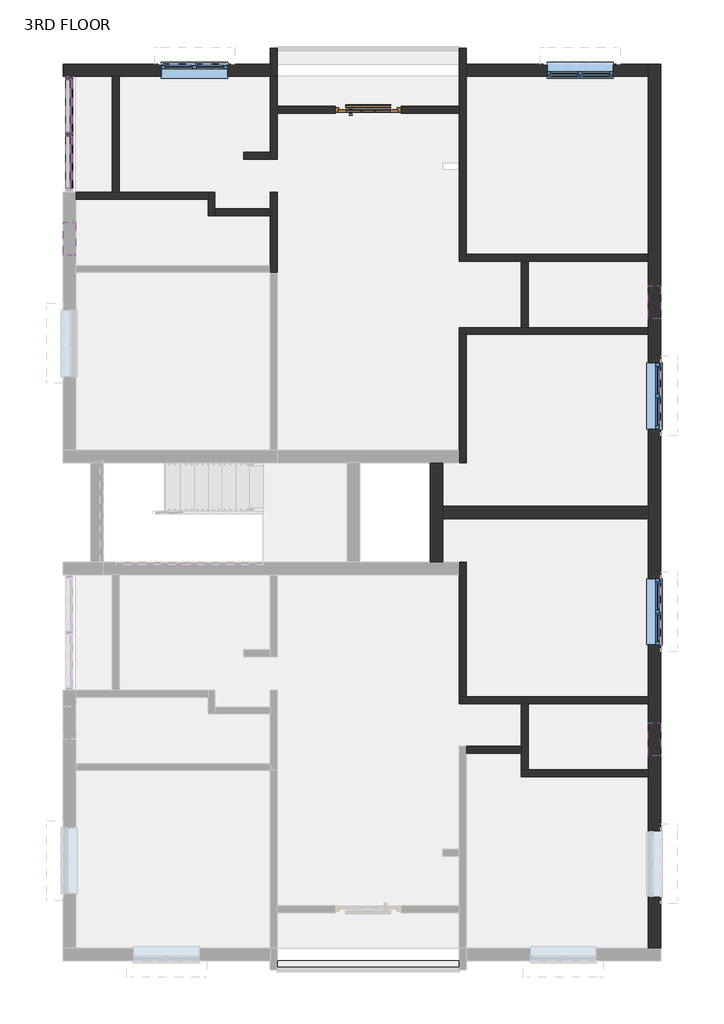
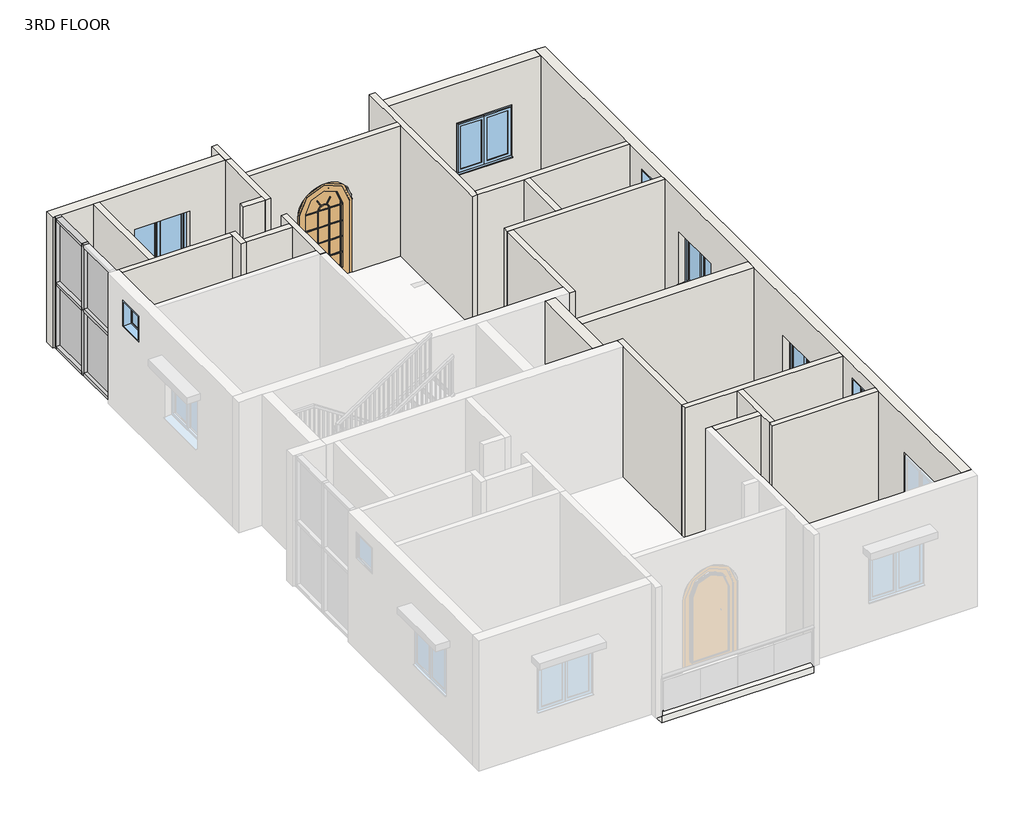
# One storey, part 2 of 4: 24 walls, 9 members, 7 windows, 4 plates, 1 door, 1 slab.
"""IFC4 building model written with IfcOpenShell, lengths in millimetres."""

from ifc_helpers import new_model, si_unit, point, frame, frame_2d, origin, place, context, project, spatial, polyline, circle_curve, trimmed, segment, composite_curve, outline, extrude, faceted_brep, transform, mapped, element, save
from components import door_arched_single_french_glass_wood_exterior_4_x_7_french_5c4dec95, member_801a2072, member_82905deb, member_88aa5c81, member_4491d118, system_panel_glazed_a8655be6, window_80340324, w2_windows_4_x_4_9dec5fc7

model = new_model("IFC4")

# Units and contexts
model_context = context("Model", 3, world=origin())
ifc_project = project(units=[si_unit("LENGTHUNIT", "METRE", prefix="MILLI")], contexts=[model_context])

# Site, building, storey
site = spatial("IfcSite", under=ifc_project)
building = spatial("IfcBuilding", under=site)
storey = spatial("IfcBuildingStorey", under=building, Name="3RD FLOOR", Elevation=12192.0)

# Door
placement = place(None, origin())
door_arched_single_french_glass_wood_exterior_4_x_7_french_shape = door_arched_single_french_glass_wood_exterior_4_x_7_french_5c4dec95(model_context)
element("IfcDoor", 1, ObjectType="Door_Arched_Single_French_Glass_Wood_Exterior : 4' x 7' french door", at=placement, inside=storey, context=model_context, shape_type="MappedRepresentation", body=[
    mapped(door_arched_single_french_glass_wood_exterior_4_x_7_french_shape, transform((-817.6012202, 12433.0309003, 12192.0), x_axis=(1.0, 0.0, 0.0), y_axis=(0.0, 1.0, 0.0), z_axis=(0.0, 0.0, 1.0))),
])

# Members
member_shape = member_801a2072(model_context)
element("IfcMember", 2, ObjectType="Rectangular Mullion : 2.5\" x 5\" rectangular", at=placement, inside=storey, context=model_context, shape_type="MappedRepresentation", body=[
    mapped(member_shape, transform((-6318.2887202, 12007.5809003, 15240.0), x_axis=(0.0, 0.0, 1.0), y_axis=(-1.0, 0.0, 0.0), z_axis=(0.0, -1.0, 0.0))),
])
element("IfcMember", 3, ObjectType="Rectangular Mullion : 2.5\" x 5\" rectangular", at=placement, inside=storey, context=model_context, shape_type="MappedRepresentation", body=[
    mapped(member_shape, transform((-6318.2887202, 12979.1309003, 12192.0), x_axis=(0.0, 0.0, -1.0), y_axis=(-1.0, 0.0, 0.0), z_axis=(0.0, 1.0, 0.0))),
])
element("IfcMember", 4, ObjectType="Rectangular Mullion : 2.5\" x 5\" rectangular", at=placement, inside=storey, context=model_context, shape_type="MappedRepresentation", body=[
    mapped(member_shape, transform((-6318.2887202, 11944.0809003, 12192.0), x_axis=(0.0, 0.0, -1.0), y_axis=(-1.0, 0.0, 0.0), z_axis=(0.0, 1.0, 0.0))),
])
member_2_shape = member_82905deb(model_context)
element("IfcMember", 5, ObjectType="Rectangular Mullion : 2.5\" x 5\" rectangular", at=placement, inside=storey, context=model_context, shape_type="MappedRepresentation", body=[
    mapped(member_2_shape, transform((-6318.2887202, 11975.8309003, 12192.0), x_axis=(0.0, -1.0, 0.0), y_axis=(-1.0, 0.0, 0.0), z_axis=(0.0, 0.0, -1.0))),
])
member_3_shape = member_88aa5c81(model_context)
element("IfcMember", 6, ObjectType="Rectangular Mullion : 2.5\" x 5\" rectangular", at=placement, inside=storey, context=model_context, shape_type="MappedRepresentation", body=[
    mapped(member_3_shape, transform((-6318.2887202, 12007.5809003, 13716.0), x_axis=(0.0, 0.0, 1.0), y_axis=(-1.0, 0.0, 0.0), z_axis=(0.0, -1.0, 0.0))),
])
element("IfcMember", 7, ObjectType="Rectangular Mullion : 2.5\" x 5\" rectangular", at=placement, inside=storey, context=model_context, shape_type="MappedRepresentation", body=[
    mapped(member_3_shape, transform((-6318.2887202, 10972.5309003, 13716.0), x_axis=(0.0, 0.0, 1.0), y_axis=(-1.0, 0.0, 0.0), z_axis=(0.0, -1.0, 0.0))),
])
element("IfcMember", 8, ObjectType="Rectangular Mullion : 2.5\" x 5\" rectangular", at=placement, inside=storey, context=model_context, shape_type="MappedRepresentation", body=[
    mapped(member_2_shape, transform((-6318.2887202, 11975.8309003, 13716.0), x_axis=(0.0, -1.0, 0.0), y_axis=(-1.0, 0.0, 0.0), z_axis=(0.0, 0.0, -1.0))),
])
member_4_shape = member_4491d118(model_context)
element("IfcMember", 9, ObjectType="Rectangular Mullion : 2.5\" x 5\" rectangular", at=placement, inside=storey, context=model_context, shape_type="MappedRepresentation", body=[
    mapped(member_4_shape, transform((-6318.2887202, 13042.6309003, 15240.0), x_axis=(0.0, 1.0, 0.0), y_axis=(-1.0, 0.0, 0.0), z_axis=(0.0, 0.0, 1.0))),
])
element("IfcMember", 10, ObjectType="Rectangular Mullion : 2.5\" x 5\" rectangular", at=placement, inside=storey, context=model_context, shape_type="MappedRepresentation", body=[
    mapped(member_4_shape, transform((-6318.2887202, 13042.6309003, 13716.0), x_axis=(0.0, 1.0, 0.0), y_axis=(-1.0, 0.0, 0.0), z_axis=(0.0, 0.0, 1.0))),
])

# Plates
system_panel_glazed_shape = system_panel_glazed_a8655be6(model_context)
element("IfcPlate", 11, ObjectType="System Panel : Glazed", at=placement, inside=storey, context=model_context, shape_type="MappedRepresentation", body=[
    mapped(system_panel_glazed_shape, transform((-6318.2887202, 12493.3559003, 12255.5), x_axis=(0.0, -1.0, 0.0), y_axis=(1.0, 0.0, 0.0), z_axis=(0.0, 0.0, 1.0))),
])
element("IfcPlate", 12, ObjectType="System Panel : Glazed", at=placement, inside=storey, context=model_context, shape_type="MappedRepresentation", body=[
    mapped(system_panel_glazed_shape, transform((-6318.2887202, 11458.3059003, 12255.5), x_axis=(0.0, -1.0, 0.0), y_axis=(1.0, 0.0, 0.0), z_axis=(0.0, 0.0, 1.0))),
])
element("IfcPlate", 13, ObjectType="System Panel : Glazed", at=placement, inside=storey, context=model_context, shape_type="MappedRepresentation", body=[
    mapped(system_panel_glazed_shape, transform((-6318.2887202, 12493.3559003, 13747.75), x_axis=(0.0, -1.0, 0.0), y_axis=(1.0, 0.0, 0.0), z_axis=(0.0, 0.0, 1.0))),
])
element("IfcPlate", 14, ObjectType="System Panel : Glazed", at=placement, inside=storey, context=model_context, shape_type="MappedRepresentation", body=[
    mapped(system_panel_glazed_shape, transform((-6318.2887202, 11458.3059003, 13747.75), x_axis=(0.0, -1.0, 0.0), y_axis=(1.0, 0.0, 0.0), z_axis=(0.0, 0.0, 1.0))),
])

# Slab
element("IfcSlab", 15, ObjectType="bathroom tiles", at=placement, inside=storey, context=model_context, shape_type="SweptSolid", body=[
    extrude(outline(polyline([(858.7987798, -3238.7690997), (858.7987798, -3403.8690997), (-2494.0012202, -3403.8690997), (-2494.0012202, -3238.7690997), (858.7987798, -3238.7690997)])), frame((0.0, 0.0, 12039.6), z_axis=(0.0, 0.0, 1.0), x_axis=(1.0, 0.0, 0.0)), (0.0, 0.0, 1.0), 152.4),
])

# Walls
element("IfcWall", 16, ObjectType="OUTER WALL 9\"", at=placement, inside=storey, context=model_context, shape_type="Brep", body=[
    faceted_brep([(4567.1987798, -3010.1690997, 12192.0), (4567.1987798, 13271.2309003, 12192.0), (4567.1987798, 13271.2309003, 15240.0), (4567.1987798, -3010.1690997, 15240.0), (4567.1987798, -844.8190997, 13192.0), (4567.1987798, -2064.0190997, 13192.0), (4567.1987798, -2064.0190997, 14411.2), (4567.1987798, -844.8190997, 14411.2), (4567.1987798, 2577.8309003, 13106.4), (4567.1987798, 2577.8309003, 14325.6), (4567.1987798, 3797.0309003, 14325.6), (4567.1987798, 3797.0309003, 13106.4), (4567.1987798, 6552.9309003, 13106.4), (4567.1987798, 6552.9309003, 14325.6), (4567.1987798, 7772.1309003, 14325.6), (4567.1987798, 7772.1309003, 13106.4), (4567.1987798, 539.4809003, 14935.2), (4567.1987798, 1149.0809003, 14935.2), (4567.1987798, 1149.0809003, 14325.6), (4567.1987798, 539.4809003, 14325.6), (4567.1987798, 8584.9309003, 14935.2), (4567.1987798, 9194.5309003, 14935.2), (4567.1987798, 9194.5309003, 14325.6), (4567.1987798, 8584.9309003, 14325.6), (4338.5987798, -3010.1690997, 12192.0), (4338.5987798, -3010.1690997, 15240.0), (4338.5987798, 152.1309003, 15240.0), (4338.5987798, 279.1309003, 15240.0), (4338.5987798, 1498.3309003, 15240.0), (4338.5987798, 1625.3309003, 15240.0), (4338.5987798, 4901.9309003, 15240.0), (4338.5987798, 5130.5309003, 15240.0), (4338.5987798, 8292.8309003, 15240.0), (4338.5987798, 8419.8309003, 15240.0), (4338.5987798, 9639.0309003, 15240.0), (4338.5987798, 9766.0309003, 15240.0), (4338.5987798, 13042.6309003, 15240.0), (4338.5987798, 13271.2309003, 15240.0), (4338.5987798, 13271.2309003, 12192.0), (4338.5987798, 13042.6309003, 12192.0), (4338.5987798, 9766.0309003, 12192.0), (4338.5987798, 9639.0309003, 12192.0), (4338.5987798, 8419.8309003, 12192.0), (4338.5987798, 8292.8309003, 12192.0), (4338.5987798, 5130.5309003, 12192.0), (4338.5987798, 4901.9309003, 12192.0), (4338.5987798, 1625.3309003, 12192.0), (4338.5987798, 1498.3309003, 12192.0), (4338.5987798, 279.1309003, 12192.0), (4338.5987798, 152.1309003, 12192.0), (4338.5987798, -844.8190997, 13192.0), (4338.5987798, -844.8190997, 14411.2), (4338.5987798, -2064.0190997, 14411.2), (4338.5987798, -2064.0190997, 13192.0), (4338.5987798, 2577.8309003, 13106.4), (4338.5987798, 3797.0309003, 13106.4), (4338.5987798, 3797.0309003, 14325.6), (4338.5987798, 2577.8309003, 14325.6), (4338.5987798, 6552.9309003, 13106.4), (4338.5987798, 7772.1309003, 13106.4), (4338.5987798, 7772.1309003, 14325.6), (4338.5987798, 6552.9309003, 14325.6), (4338.5987798, 539.4809003, 14935.2), (4338.5987798, 539.4809003, 14325.6), (4338.5987798, 1149.0809003, 14325.6), (4338.5987798, 1149.0809003, 14935.2), (4338.5987798, 8584.9309003, 14935.2), (4338.5987798, 8584.9309003, 14325.6), (4338.5987798, 9194.5309003, 14325.6), (4338.5987798, 9194.5309003, 14935.2)], [[[0, 1, 2, 3], [4, 5, 6, 7], [8, 9, 10, 11], [12, 13, 14, 15], [16, 17, 18, 19], [20, 21, 22, 23]], [[24, 25, 26, 27, 28, 29, 30, 31, 32, 33, 34, 35, 36, 37, 38, 39, 40, 41, 42, 43, 44, 45, 46, 47, 48, 49], [50, 51, 52, 53], [54, 55, 56, 57], [58, 59, 60, 61], [62, 63, 64, 65], [66, 67, 68, 69]], [[1, 0, 24, 49, 48, 47, 46, 45, 44, 43, 42, 41, 40, 39, 38]], [[3, 2, 37, 36, 35, 34, 33, 32, 31, 30, 29, 28, 27, 26, 25]], [[0, 3, 25, 24]], [[2, 1, 38, 37]], [[51, 50, 4, 7]], [[52, 51, 7, 6]], [[53, 52, 6, 5]], [[50, 53, 5, 4]], [[9, 8, 54, 57]], [[10, 9, 57, 56]], [[11, 10, 56, 55]], [[8, 11, 55, 54]], [[13, 12, 58, 61]], [[14, 13, 61, 60]], [[15, 14, 60, 59]], [[12, 15, 59, 58]], [[63, 62, 16, 19]], [[64, 63, 19, 18]], [[65, 64, 18, 17]], [[62, 65, 17, 16]], [[67, 66, 20, 23]], [[68, 67, 23, 22]], [[69, 68, 22, 21]], [[66, 69, 21, 20]]]),
])
element("IfcWall", 17, ObjectType="OUTER WALL 9\"", at=placement, inside=storey, context=model_context, shape_type="SweptSolid", body=[
    extrude(outline(polyline([(12192.0, 4338.5987798), (15240.0, 4338.5987798), (15240.0, 985.7987798), (12192.0, 985.7987798), (12192.0, 4338.5987798)]), holes=[polyline([(13106.4, 2479.7847416), (14325.6, 2479.7847416), (14325.6, 3698.9847416), (13106.4, 3698.9847416), (13106.4, 2479.7847416)])]), frame((0.0, 13042.6309003, 0.0), z_axis=(0.0, 1.0, 0.0), x_axis=(0.0, 0.0, 1.0)), (0.0, 0.0, 1.0), 228.6),
])
element("IfcWall", 18, ObjectType="OUTER WALL 9\"", at=placement, inside=storey, context=model_context, shape_type="Brep", body=[
    faceted_brep([(-2621.0012202, 13271.2309003, 12192.0), (-6432.5887202, 13271.2309003, 12192.0), (-6432.5887202, 13271.2309003, 15240.0), (-2621.0012202, 13271.2309003, 15240.0), (-3402.0512202, 13271.2309003, 13106.4), (-3402.0512202, 13271.2309003, 14325.6), (-4621.2512202, 13271.2309003, 14325.6), (-4621.2512202, 13271.2309003, 13106.4), (-2621.0012202, 13042.6309003, 12192.0), (-2621.0012202, 13042.6309003, 15240.0), (-5402.3012202, 13042.6309003, 15240.0), (-5529.3012202, 13042.6309003, 15240.0), (-6432.5887202, 13042.6309003, 15240.0), (-6432.5887202, 13042.6309003, 12192.0), (-5529.3012202, 13042.6309003, 12192.0), (-5402.3012202, 13042.6309003, 12192.0), (-3402.0512202, 13042.6309003, 13106.4), (-4621.2512202, 13042.6309003, 13106.4), (-4621.2512202, 13042.6309003, 14325.6), (-3402.0512202, 13042.6309003, 14325.6)], [[[0, 1, 2, 3], [4, 5, 6, 7]], [[8, 9, 10, 11, 12, 13, 14, 15], [16, 17, 18, 19]], [[1, 0, 8, 15, 14, 13]], [[3, 2, 12, 11, 10, 9]], [[2, 1, 13, 12]], [[5, 4, 16, 19]], [[6, 5, 19, 18]], [[7, 6, 18, 17]], [[4, 7, 17, 16]], [[0, 3, 9, 8]]]),
])
element("IfcWall", 19, ObjectType="OUTER WALL 9\"", at=placement, inside=storey, context=model_context, shape_type="Brep", body=[
    faceted_brep([(553.9987798, 4101.8309003, 12192.0), (553.9987798, 4901.9309003, 12192.0), (553.9987798, 5130.5309003, 12192.0), (553.9987798, 5930.6309003, 12192.0), (553.9987798, 5930.6309003, 15240.0), (553.9987798, 5130.5309003, 15240.0), (553.9987798, 4901.9309003, 15240.0), (553.9987798, 4101.8309003, 15240.0), (325.3987798, 4101.8309003, 12192.0), (325.3987798, 4101.8309003, 15240.0), (325.3987798, 5930.6309003, 15240.0), (325.3987798, 5930.6309003, 12192.0)], [[[0, 1, 2, 3, 4, 5, 6, 7]], [[8, 9, 10, 11]], [[3, 2, 1, 0, 8, 11]], [[7, 6, 5, 4, 10, 9]], [[0, 7, 9, 8]], [[4, 3, 11, 10]]]),
])
element("IfcWall", 20, ObjectType="OUTER WALL 9\"", at=placement, inside=storey, context=model_context, shape_type="SweptSolid", body=[
    extrude(outline(polyline([(4338.5987798, 4901.9309003), (553.9987798, 4901.9309003), (553.9987798, 5130.5309003), (4338.5987798, 5130.5309003), (4338.5987798, 4901.9309003)])), frame((0.0, 0.0, 12192.0), z_axis=(0.0, 0.0, 1.0), x_axis=(1.0, 0.0, 0.0)), (0.0, 0.0, 1.0), 3048.0),
])
element("IfcWall", 21, ObjectType="inner wall 5\"", at=placement, inside=storey, context=model_context, shape_type="SweptSolid", body=[
    extrude(outline(polyline([(-5529.3012202, 10909.0309003), (-5529.3012202, 13042.6309003), (-5402.3012202, 13042.6309003), (-5402.3012202, 10909.0309003), (-5529.3012202, 10909.0309003)])), frame((0.0, 0.0, 12192.0), z_axis=(0.0, 0.0, 1.0), x_axis=(1.0, 0.0, 0.0)), (0.0, 0.0, 1.0), 3048.0),
])
element("IfcWall", 22, ObjectType="inner wall 5\"", at=placement, inside=storey, context=model_context, shape_type="Brep", body=[
    faceted_brep([(-2621.0012202, 13042.6309003, 12192.0), (-2621.0012202, 11645.6309003, 12192.0), (-2621.0012202, 11518.6309003, 12192.0), (-2621.0012202, 11518.6309003, 15240.0), (-2621.0012202, 11645.6309003, 15240.0), (-2621.0012202, 13042.6309003, 15240.0), (-2494.0012202, 13042.6309003, 12192.0), (-2494.0012202, 13042.6309003, 15240.0), (-2494.0012202, 12496.5309003, 15240.0), (-2494.0012202, 12369.5309003, 15240.0), (-2494.0012202, 11518.6309003, 15240.0), (-2494.0012202, 11518.6309003, 12192.0), (-2494.0012202, 12369.5309003, 12192.0), (-2494.0012202, 12496.5309003, 12192.0)], [[[0, 1, 2, 3, 4, 5]], [[6, 7, 8, 9, 10, 11, 12, 13]], [[2, 1, 0, 6, 13, 12, 11]], [[5, 4, 3, 10, 9, 8, 7]], [[3, 2, 11, 10]], [[0, 5, 7, 6]]]),
])
element("IfcWall", 23, ObjectType="inner wall 5\"", at=placement, inside=storey, context=model_context, shape_type="SweptSolid", body=[
    extrude(outline(polyline([(-3103.6012202, 11645.6309003), (-2621.0012202, 11645.6309003), (-2621.0012202, 11518.6309003), (-3103.6012202, 11518.6309003), (-3103.6012202, 11645.6309003)])), frame((0.0, 0.0, 12192.0), z_axis=(0.0, 0.0, 1.0), x_axis=(1.0, 0.0, 0.0)), (0.0, 0.0, 1.0), 3048.0),
])
element("IfcWall", 24, ObjectType="inner wall 5\"", at=placement, inside=storey, context=model_context, shape_type="Brep", body=[
    faceted_brep([(-6202.4012202, 10782.0309003, 12192.0), (-3764.0012202, 10782.0309003, 12192.0), (-3764.0012202, 10782.0309003, 15240.0), (-6202.4012202, 10782.0309003, 15240.0), (-6202.4012202, 10909.0309003, 12192.0), (-6202.4012202, 10909.0309003, 15240.0), (-5529.3012202, 10909.0309003, 15240.0), (-5402.3012202, 10909.0309003, 15240.0), (-3764.0012202, 10909.0309003, 15240.0), (-3764.0012202, 10909.0309003, 12192.0), (-5402.3012202, 10909.0309003, 12192.0), (-5529.3012202, 10909.0309003, 12192.0)], [[[0, 1, 2, 3]], [[4, 5, 6, 7, 8, 9, 10, 11]], [[1, 0, 4, 11, 10, 9]], [[3, 2, 8, 7, 6, 5]], [[0, 3, 5, 4]], [[2, 1, 9, 8]]]),
])
element("IfcWall", 25, ObjectType="inner wall 5\"", at=placement, inside=storey, context=model_context, shape_type="Brep", body=[
    faceted_brep([(-3764.0012202, 10909.0309003, 12192.0), (-3764.0012202, 10782.0309003, 12192.0), (-3764.0012202, 10477.2309003, 12192.0), (-3764.0012202, 10477.2309003, 15240.0), (-3764.0012202, 10782.0309003, 15240.0), (-3764.0012202, 10909.0309003, 15240.0), (-3637.0012202, 10909.0309003, 12192.0), (-3637.0012202, 10909.0309003, 15240.0), (-3637.0012202, 10604.2309003, 15240.0), (-3637.0012202, 10477.2309003, 15240.0), (-3637.0012202, 10477.2309003, 12192.0), (-3637.0012202, 10604.2309003, 12192.0)], [[[0, 1, 2, 3, 4, 5]], [[6, 7, 8, 9, 10, 11]], [[2, 1, 0, 6, 11, 10]], [[5, 4, 3, 9, 8, 7]], [[0, 5, 7, 6]], [[3, 2, 10, 9]]]),
])
element("IfcWall", 26, ObjectType="inner wall 5\"", at=placement, inside=storey, context=model_context, shape_type="SweptSolid", body=[
    extrude(outline(polyline([(-2621.0012202, 10477.2309003), (-3637.0012202, 10477.2309003), (-3637.0012202, 10604.2309003), (-2621.0012202, 10604.2309003), (-2621.0012202, 10477.2309003)])), frame((0.0, 0.0, 12192.0), z_axis=(0.0, 0.0, 1.0), x_axis=(1.0, 0.0, 0.0)), (0.0, 0.0, 1.0), 3048.0),
])
element("IfcWall", 27, ObjectType="inner wall 5\"", at=placement, inside=storey, context=model_context, shape_type="Brep", body=[
    faceted_brep([(-2621.0012202, 10909.0309003, 12192.0), (-2621.0012202, 10604.2309003, 12192.0), (-2621.0012202, 10477.2309003, 12192.0), (-2621.0012202, 9562.8309003, 12192.0), (-2621.0012202, 9435.8309003, 12192.0), (-2621.0012202, 9435.8309003, 15240.0), (-2621.0012202, 9562.8309003, 15240.0), (-2621.0012202, 10477.2309003, 15240.0), (-2621.0012202, 10604.2309003, 15240.0), (-2621.0012202, 10909.0309003, 15240.0), (-2494.0012202, 10909.0309003, 12192.0), (-2494.0012202, 10909.0309003, 15240.0), (-2494.0012202, 9435.8309003, 15240.0), (-2494.0012202, 9435.8309003, 12192.0)], [[[0, 1, 2, 3, 4, 5, 6, 7, 8, 9]], [[10, 11, 12, 13]], [[4, 3, 2, 1, 0, 10, 13]], [[9, 8, 7, 6, 5, 12, 11]], [[0, 9, 11, 10]], [[5, 4, 13, 12]]]),
])
element("IfcWall", 28, ObjectType="inner wall 5\"", at=placement, inside=storey, context=model_context, shape_type="SweptSolid", body=[
    extrude(outline(polyline([(2001.7987798, 583.9309003), (985.7987798, 583.9309003), (985.7987798, 710.9309003), (2001.7987798, 710.9309003), (2001.7987798, 583.9309003)])), frame((0.0, 0.0, 12192.0), z_axis=(0.0, 0.0, 1.0), x_axis=(1.0, 0.0, 0.0)), (0.0, 0.0, 1.0), 3048.0),
])
element("IfcWall", 29, ObjectType="inner wall 5\"", at=placement, inside=storey, context=model_context, shape_type="Brep", body=[
    faceted_brep([(4338.5987798, 1625.3309003, 12192.0), (985.7987798, 1625.3309003, 12192.0), (858.7987798, 1625.3309003, 12192.0), (858.7987798, 1625.3309003, 15240.0), (985.7987798, 1625.3309003, 15240.0), (4338.5987798, 1625.3309003, 15240.0), (4338.5987798, 1498.3309003, 12192.0), (4338.5987798, 1498.3309003, 15240.0), (2128.7987798, 1498.3309003, 15240.0), (2001.7987798, 1498.3309003, 15240.0), (858.7987798, 1498.3309003, 15240.0), (858.7987798, 1498.3309003, 12192.0), (2001.7987798, 1498.3309003, 12192.0), (2128.7987798, 1498.3309003, 12192.0)], [[[0, 1, 2, 3, 4, 5]], [[6, 7, 8, 9, 10, 11, 12, 13]], [[2, 1, 0, 6, 13, 12, 11]], [[5, 4, 3, 10, 9, 8, 7]], [[3, 2, 11, 10]], [[0, 5, 7, 6]]]),
])
element("IfcWall", 30, ObjectType="inner wall 5\"", at=placement, inside=storey, context=model_context, shape_type="Brep", body=[
    faceted_brep([(985.7987798, 1625.3309003, 12192.0), (985.7987798, 4101.8309003, 12192.0), (985.7987798, 4101.8309003, 15240.0), (985.7987798, 1625.3309003, 15240.0), (858.7987798, 1625.3309003, 12192.0), (858.7987798, 1625.3309003, 15240.0), (858.7987798, 3873.2309003, 15240.0), (858.7987798, 4101.8309003, 15240.0), (858.7987798, 4101.8309003, 12192.0), (858.7987798, 3873.2309003, 12192.0)], [[[0, 1, 2, 3]], [[4, 5, 6, 7, 8, 9]], [[1, 0, 4, 9, 8]], [[3, 2, 7, 6, 5]], [[0, 3, 5, 4]], [[2, 1, 8, 7]]]),
])
element("IfcWall", 31, ObjectType="inner wall 5\"", at=placement, inside=storey, context=model_context, shape_type="Brep", body=[
    faceted_brep([(4338.5987798, 279.1309003, 12192.0), (2128.7987798, 279.1309003, 12192.0), (2001.7987798, 279.1309003, 12192.0), (2001.7987798, 279.1309003, 15240.0), (2128.7987798, 279.1309003, 15240.0), (4338.5987798, 279.1309003, 15240.0), (4338.5987798, 152.1309003, 12192.0), (4338.5987798, 152.1309003, 15240.0), (2001.7987798, 152.1309003, 15240.0), (2001.7987798, 152.1309003, 12192.0)], [[[0, 1, 2, 3, 4, 5]], [[6, 7, 8, 9]], [[2, 1, 0, 6, 9]], [[5, 4, 3, 8, 7]], [[0, 5, 7, 6]], [[3, 2, 9, 8]]]),
])
element("IfcWall", 32, ObjectType="inner wall 5\"", at=placement, inside=storey, context=model_context, shape_type="Brep", body=[
    faceted_brep([(2128.7987798, 279.1309003, 12192.0), (2128.7987798, 1498.3309003, 12192.0), (2128.7987798, 1498.3309003, 15240.0), (2128.7987798, 279.1309003, 15240.0), (2001.7987798, 279.1309003, 12192.0), (2001.7987798, 279.1309003, 15240.0), (2001.7987798, 583.9309003, 15240.0), (2001.7987798, 710.9309003, 15240.0), (2001.7987798, 1498.3309003, 15240.0), (2001.7987798, 1498.3309003, 12192.0), (2001.7987798, 710.9309003, 12192.0), (2001.7987798, 583.9309003, 12192.0)], [[[0, 1, 2, 3]], [[4, 5, 6, 7, 8, 9, 10, 11]], [[1, 0, 4, 11, 10, 9]], [[3, 2, 8, 7, 6, 5]], [[0, 3, 5, 4]], [[2, 1, 9, 8]]]),
])
element("IfcWall", 33, ObjectType="inner wall 5\"", at=placement, inside=storey, context=model_context, shape_type="SweptSolid", body=[
    extrude(outline(composite_curve([segment(polyline([(13870.6, -208.0012202), (12192.0, -208.0012202), (12192.0, 858.7987798), (15240.0, 858.7987798), (15240.0, -2494.0012202), (12192.0, -2494.0012202), (12192.0, -1427.2012202), (13870.6, -1427.2012202)]), True, "CONTINUOUS"), segment(trimmed(circle_curve(frame_2d((13870.6, -817.6012202)), 609.6), [point((13870.6, -1427.2012202))], [point((13870.6, -208.0012202))], True, "CARTESIAN"), True, "CONTINUOUS")], self_intersect=False)), frame((0.0, 12369.5309003, 0.0), z_axis=(0.0, 1.0, 0.0), x_axis=(0.0, 0.0, 1.0)), (0.0, 0.0, 1.0), 127.0),
])
element("IfcWall", 34, ObjectType="inner wall 5\"", at=placement, inside=storey, context=model_context, shape_type="Brep", body=[
    faceted_brep([(858.7987798, 13563.3309003, 12192.0), (858.7987798, 12496.5309003, 12192.0), (858.7987798, 12369.5309003, 12192.0), (858.7987798, 9639.0309003, 12192.0), (858.7987798, 9639.0309003, 15240.0), (858.7987798, 12369.5309003, 15240.0), (858.7987798, 12496.5309003, 15240.0), (858.7987798, 13563.3309003, 15240.0), (985.7987798, 13563.3309003, 12192.0), (985.7987798, 13563.3309003, 15240.0), (985.7987798, 13271.2309003, 15240.0), (985.7987798, 13042.6309003, 15240.0), (985.7987798, 9766.0309003, 15240.0), (985.7987798, 9639.0309003, 15240.0), (985.7987798, 9639.0309003, 12192.0), (985.7987798, 9766.0309003, 12192.0), (985.7987798, 13042.6309003, 12192.0), (985.7987798, 13271.2309003, 12192.0)], [[[0, 1, 2, 3, 4, 5, 6, 7]], [[8, 9, 10, 11, 12, 13, 14, 15, 16, 17]], [[3, 2, 1, 0, 8, 17, 16, 15, 14]], [[7, 6, 5, 4, 13, 12, 11, 10, 9]], [[0, 7, 9, 8]], [[4, 3, 14, 13]]]),
])
element("IfcWall", 35, ObjectType="inner wall 5\"", at=placement, inside=storey, context=model_context, shape_type="Brep", body=[
    faceted_brep([(4338.5987798, 9766.0309003, 12192.0), (985.7987798, 9766.0309003, 12192.0), (985.7987798, 9766.0309003, 15240.0), (4338.5987798, 9766.0309003, 15240.0), (4338.5987798, 9639.0309003, 12192.0), (4338.5987798, 9639.0309003, 15240.0), (2128.7987798, 9639.0309003, 15240.0), (2001.7987798, 9639.0309003, 15240.0), (985.7987798, 9639.0309003, 15240.0), (985.7987798, 9639.0309003, 12192.0), (2001.7987798, 9639.0309003, 12192.0), (2128.7987798, 9639.0309003, 12192.0)], [[[0, 1, 2, 3]], [[4, 5, 6, 7, 8, 9, 10, 11]], [[1, 0, 4, 11, 10, 9]], [[3, 2, 8, 7, 6, 5]], [[0, 3, 5, 4]], [[2, 1, 9, 8]]]),
])
element("IfcWall", 36, ObjectType="inner wall 5\"", at=placement, inside=storey, context=model_context, shape_type="Brep", body=[
    faceted_brep([(4338.5987798, 8419.8309003, 12192.0), (2128.7987798, 8419.8309003, 12192.0), (2001.7987798, 8419.8309003, 12192.0), (858.7987798, 8419.8309003, 12192.0), (858.7987798, 8419.8309003, 15240.0), (2001.7987798, 8419.8309003, 15240.0), (2128.7987798, 8419.8309003, 15240.0), (4338.5987798, 8419.8309003, 15240.0), (4338.5987798, 8292.8309003, 12192.0), (4338.5987798, 8292.8309003, 15240.0), (985.7987798, 8292.8309003, 15240.0), (858.7987798, 8292.8309003, 15240.0), (858.7987798, 8292.8309003, 12192.0), (985.7987798, 8292.8309003, 12192.0)], [[[0, 1, 2, 3, 4, 5, 6, 7]], [[8, 9, 10, 11, 12, 13]], [[3, 2, 1, 0, 8, 13, 12]], [[7, 6, 5, 4, 11, 10, 9]], [[0, 7, 9, 8]], [[4, 3, 12, 11]]]),
])
element("IfcWall", 37, ObjectType="inner wall 5\"", at=placement, inside=storey, context=model_context, shape_type="SweptSolid", body=[
    extrude(outline(polyline([(2128.7987798, 9639.0309003), (2128.7987798, 8419.8309003), (2001.7987798, 8419.8309003), (2001.7987798, 9639.0309003), (2128.7987798, 9639.0309003)])), frame((0.0, 0.0, 12192.0), z_axis=(0.0, 0.0, 1.0), x_axis=(1.0, 0.0, 0.0)), (0.0, 0.0, 1.0), 3048.0),
])
element("IfcWall", 38, ObjectType="inner wall 5\"", at=placement, inside=storey, context=model_context, shape_type="Brep", body=[
    faceted_brep([(858.7987798, 8292.8309003, 12192.0), (858.7987798, 6159.2309003, 12192.0), (858.7987798, 5930.6309003, 12192.0), (858.7987798, 5930.6309003, 15240.0), (858.7987798, 6159.2309003, 15240.0), (858.7987798, 8292.8309003, 15240.0), (985.7987798, 8292.8309003, 12192.0), (985.7987798, 8292.8309003, 15240.0), (985.7987798, 5930.6309003, 15240.0), (985.7987798, 5930.6309003, 12192.0)], [[[0, 1, 2, 3, 4, 5]], [[6, 7, 8, 9]], [[2, 1, 0, 6, 9]], [[5, 4, 3, 8, 7]], [[0, 5, 7, 6]], [[3, 2, 9, 8]]]),
])
element("IfcWall", 39, ObjectType="inner wall 5\"", at=placement, inside=storey, context=model_context, shape_type="Brep", body=[
    faceted_brep([(-2494.0012202, 13042.6309003, 12192.0), (-2494.0012202, 13563.3309003, 12192.0), (-2494.0012202, 13563.3309003, 15240.0), (-2494.0012202, 13042.6309003, 15240.0), (-2621.0012202, 13042.6309003, 12192.0), (-2621.0012202, 13042.6309003, 15240.0), (-2621.0012202, 13271.2309003, 15240.0), (-2621.0012202, 13563.3309003, 15240.0), (-2621.0012202, 13563.3309003, 12192.0), (-2621.0012202, 13271.2309003, 12192.0)], [[[0, 1, 2, 3]], [[4, 5, 6, 7, 8, 9]], [[1, 0, 4, 9, 8]], [[2, 1, 8, 7]], [[3, 2, 7, 6, 5]], [[0, 3, 5, 4]]]),
])

# Windows
window_shape = window_80340324(model_context)
element("IfcWindow", 40, ObjectType="Fixed : 24\" x 24\"", at=placement, inside=storey, context=model_context, shape_type="MappedRepresentation", body=[
    mapped(window_shape, transform((4452.8987798, 8851.6309003, 13411.2), x_axis=(0.0, -1.0, 0.0), y_axis=(1.0, 0.0, 0.0), z_axis=(0.0, 0.0, 1.0))),
])
element("IfcWindow", 41, ObjectType="Fixed : 24\" x 24\"", at=placement, inside=storey, context=model_context, shape_type="MappedRepresentation", body=[
    mapped(window_shape, transform((4452.8987798, 806.1809003, 13411.2), x_axis=(0.0, -1.0, 0.0), y_axis=(1.0, 0.0, 0.0), z_axis=(0.0, 0.0, 1.0))),
])
element("IfcWindow", 42, ObjectType="Fixed : 24\" x 24\"", at=placement, inside=storey, context=model_context, shape_type="MappedRepresentation", body=[
    mapped(window_shape, transform((-6318.2887202, 10020.0309003, 13411.2), x_axis=(0.0, -1.0, 0.0), y_axis=(1.0, 0.0, 0.0), z_axis=(0.0, 0.0, 1.0))),
])
w2_windows_4_x_4_shape = w2_windows_4_x_4_9dec5fc7(model_context)
element("IfcWindow", 43, ObjectType="w2 : windows 4' x 4'", at=placement, inside=storey, context=model_context, shape_type="MappedRepresentation", body=[
    mapped(w2_windows_4_x_4_shape, transform((3089.3847416, 13156.9309003, 12106.4), x_axis=(1.0, 0.0, 0.0), y_axis=(0.0, 1.0, 0.0), z_axis=(0.0, 0.0, 1.0))),
])
element("IfcWindow", 44, ObjectType="w2 : windows 4' x 4'", at=placement, inside=storey, context=model_context, shape_type="MappedRepresentation", body=[
    mapped(w2_windows_4_x_4_shape, transform((-4011.6512202, 13156.9309003, 12106.4), x_axis=(-1.0, 0.0, 0.0), y_axis=(0.0, -1.0, 0.0), z_axis=(0.0, 0.0, 1.0))),
])
element("IfcWindow", 45, ObjectType="w2 : windows 4' x 4'", at=placement, inside=storey, context=model_context, shape_type="MappedRepresentation", body=[
    mapped(w2_windows_4_x_4_shape, transform((4452.8987798, 7162.5309003, 12106.4), x_axis=(0.0, 1.0, 0.0), y_axis=(-1.0, 0.0, 0.0), z_axis=(0.0, 0.0, 1.0))),
])
element("IfcWindow", 46, ObjectType="w2 : windows 4' x 4'", at=placement, inside=storey, context=model_context, shape_type="MappedRepresentation", body=[
    mapped(w2_windows_4_x_4_shape, transform((4452.8987798, 3187.4309003, 12106.4), x_axis=(0.0, 1.0, 0.0), y_axis=(-1.0, 0.0, 0.0), z_axis=(0.0, 0.0, 1.0))),
])

save(model, "model.ifc")

# Revit data of these elements
# Type "Door_Arched_Single_French_Glass_Wood_Exterior : 4' x 7' french door"
#   Type Mark = "17"
#   Type Comments = "External Single"
#   Operation = "SingleSwingRight"
#   Keynote = "L20"
#   Analytic Construction = "<None>"
#   Wrap Layers (Int) from Ext = 0' - 6.98819"
#   Wrap Layers (Ext) from Ext = 0' - 4.03543"
#   Thickness = 0' - 1.73228"
#   Stile Shutting = 0' - 5.90551"
#   Stile - Top Rail = 0' - 5.90551"
#   Stile - Hanging = 0' - 5.90551"
#   Stile - Bottom Rail = 0' - 6.88976"
#   Rough Width = 4' - 0"
#   Rough Height = 7' - 0"
#   O/A Frame Width = 0' - 2.51969"
#   Handle Z Distance = 3' - 5.33858"
#   Glazing Thickness = 0' - 0.94488"
#   Glazing Bar Thickness = 0' - 0.7874"
#   FrameWidth = 0' - 1.65354"
#   FrameOffset - External = 0' - 0.98425"
#   FrameDepth = 0' - 3.50394"
#   Door Panel Width = 3' - 7.94488"
#   Handle X Distance = 0' - 2.95276"
#   Height = 7' - 0"
#   Structural Tolerance = 0' - 0.25591"
#   Tolerance = 0' - 0.11811"
#   Undercut = 0' - 0.15748"
#   Width = 4' - 0"
#   Door Panel Thickness = 0' - 1.73228"
#   Door Panel Height = 6' - 9.81496"
#   Cavity Closer Width = 0' - 1.9685"
#   Cavity Closer Offset from Ext = 0' - 4.03543"
#   Cavity Closer Depth = 0' - 3.34646"
#   Vis - Ironmongery = yes
#   Vis - Cavity Closers = yes
#   Define Thermal Properties by = 1
#   Material Glass = Door - Glazing
#   Handle Style = element 430241
#   Material Door = Door - Panel
#   Material Frame = BROWN
#   Material Ironmongery = Door - Handle
#   Function = (empty or 0)
#   Wall Closure = (empty or 0)
#   Assembly Code = ""
# Type "Rectangular Mullion : 2.5\" x 5\" rectangular"
#   built-in parameter 1007304 = 0.416667 (stored number, unit not read)
#   built-in parameter 1007301 = 0.104167 (stored number, unit not read)
#   built-in parameter 1007300 = 0.104167 (stored number, unit not read)
# Type "System Panel : Glazed"
#   Construction Type Id = "GSP4R"
#   Analytic Construction = "1/8 in Pilkington single glazing"
#   Visual Light Transmittance = 0.9
#   Solar Heat Gain Coefficient = 0.86
#   Heat Transfer Coefficient (U) = 1.18115 BTU/(h·ft²·°F)
#   Define Thermal Properties by = 1
# Type "bathroom tiles"
#   Assembly Code = "B1010"
#   Function = 0
#   Layers, outside or top first: 0' - 6" "tile flooring" (function 1)
# Type "OUTER WALL 9\""
#   Assembly Code = "B2010"
#   Layers, outside or top first: 0' - 9" "ROSE COLOUR" (function 1)
# Type "inner wall 5\""
#   Assembly Code = "B2010"
#   Layers, outside or top first: 0' - 5" "ROSE COLOUR" (function 1)
# Type "Fixed : 24\" x 24\""
#   Type Mark = "3"
#   Construction Type Id = "GSP4R"
#   Assembly Code = "B2020100"
#   Analytic Construction = "1/8 in Pilkington single glazing"
#   Visual Light Transmittance = 0.9
#   Solar Heat Gain Coefficient = 0.78
#   Heat Transfer Coefficient (U) = 0.6496 BTU/(h·ft²·°F)
#   Height = 2' - 0"
#   Default Sill Height = 3' - 0"
#   Width = 2' - 0"
#   Window Inset = 0' - 0 3/4"
#   Define Thermal Properties by = 1
#   Define Thermal Properties by = 1
#   Glass Pane Material = Glass
#   Sash Material = Sash
#   Wall Closure = (empty or 0)
# Type "w2 : windows 4' x 4'"
#   Type Mark = "31"
#   Operation = "DoublePanelVertical"
#   Keynote = "16.05.01"
#   Analytic Construction = "<None>"
#   Rough Width = 4' - 0"
#   Rough Height = 4' - 0"
#   Rahmentiefe = 0' - 2.3622"
#   Rahmenhöhe unten = 0' - 3.14961"
#   Rahmehöhe oben = 0' - 3.14961"
#   Rahmenbreite = 0' - 2.3622"
#   Heat Transfer Coefficient (U) = 2.81836 BTU/(h·ft²·°F)
#   Height = 4' - 0"
#   Flügeltiefe = 0' - 2.3622"
#   Flügelbreite = 0' - 2.3622"
#   Einbautiefe (von außen) [instance default] = 0' - 5.51181"
#   Width = 4' - 0"
#   Kippflügel [instance default] = yes
#   Drehflügel im Grundriß darstellen [instance default] = no
#   Drehflügel [instance default] = yes
#   Define Thermal Properties by = 1
#   Rahmen [instance default] = none
#   Glas [instance default] = blue glass
#   Flügel [instance default] = WINDOW COLOUR WHITE
#   Fensterbank aussen [instance default] = WINDOW COLOUR WHITE
#   Fensterbank innen [instance default] = WINDOW COLOUR WHITE
#   Visual Light Transmittance = 0
#   Thermal Resistance (R) = 0
#   Solar Heat Gain Coefficient = 0
#   Wall Closure = (empty or 0)
# Element 1 (IfcDoor, "Door_Arched_Single_French_Glass_Wood_Exterior : 4' x 7' french door")
#   Phase Created = New Construction
#   Materials on its faces: "Door - Panel", "Door - Handle", "BROWN", "Door - Glazing"
# Elements 2, 3, 4, 5, 6, 7, 8, 9, 10 (IfcMember, "Rectangular Mullion : 2.5\" x 5\" rectangular")
#   Phase Created = New Construction
#   Materials on its faces: "Aluminum"
# Elements 11, 12, 13, 14 (IfcPlate, "System Panel : Glazed")
#   Phase Created = New Construction
#   Materials on its faces: "Glass"
# Element 15 (IfcSlab, "bathroom tiles")
#   Height Offset From Level = 0' - 0"
#   Phase Created = New Construction
#   Materials on its faces: "tile flooring"
# Elements 16, 17, 18, 19, 20 (IfcWall, "OUTER WALL 9\"")
#   Top Offset = 0' - 0"
#   Base Offset = 0' - 0"
#   wall height = 10' - 0"
#   Phase Created = New Construction
#   Base Constraint = 3RD FLOOR
#   Top Constraint = 4RTH FLOOR
#   Materials on its faces: "ROSE COLOUR"
# Elements 21, 22, 23, 24, 25, 26, 27, 28, 29, 30, 31, 32, 33, 34, 35, 36, 37, 38, 39 (IfcWall, "inner wall 5\"")
#   Top Offset = 0' - 0"
#   Base Offset = 0' - 0"
#   wall height = 10' - 0"
#   Phase Created = New Construction
#   Base Constraint = 3RD FLOOR
#   Top Constraint = 4RTH FLOOR
#   Materials on its faces: "ROSE COLOUR"
# Element 40 (IfcWindow, "Fixed : 24\" x 24\"")
#   Mark = "63"
#   Phase Created = New Construction
#   Materials on its faces: "Sash", "Glass"
# Element 41 (IfcWindow, "Fixed : 24\" x 24\"")
#   Mark = "65"
#   Phase Created = New Construction
#   Materials on its faces: "Sash", "Glass"
# Element 42 (IfcWindow, "Fixed : 24\" x 24\"")
#   Mark = "66"
#   Phase Created = New Construction
#   Materials on its faces: "Sash", "Glass"
# Element 43 (IfcWindow, "w2 : windows 4' x 4'")
#   Mark = "54"
#   Phase Created = New Construction
#   Materials on its faces: "WINDOW COLOUR WHITE", "blue glass"
# Element 44 (IfcWindow, "w2 : windows 4' x 4'")
#   Mark = "55"
#   Phase Created = New Construction
#   Materials on its faces: "WINDOW COLOUR WHITE", "blue glass"
# Element 45 (IfcWindow, "w2 : windows 4' x 4'")
#   Mark = "58"
#   Phase Created = New Construction
#   Materials on its faces: "WINDOW COLOUR WHITE", "blue glass"
# Element 46 (IfcWindow, "w2 : windows 4' x 4'")
#   Mark = "59"
#   Phase Created = New Construction
#   Materials on its faces: "WINDOW COLOUR WHITE", "blue glass"
# Materials
#   "Door - Glazing": colour RGB 218 227 224, transparency 0.85
#   "Door - Panel": class "Wood", colour RGB 210 159 95, transparency 0, Cost = 0
#   "BROWN": class "Generic", colour RGB 120 120 120, transparency 0, Cost = 0
#   "Door - Handle": colour RGB 0 0 0, transparency 0, Keynote = "P21"
#   "tile flooring": class "Generic", colour RGB 120 120 120, transparency 0, Cost = 0
#   "ROSE COLOUR": class "Generic", colour RGB 120 120 120, transparency 0, Cost = 0
#   "Glass": class "Glass", colour RGB 0 128 192, transparency 0.75, Description = "Soda Lime Glass", Cost = 0
#   "Sash": class "Wood", colour RGB 224 178 126, transparency 0, Cost = 0
#   "blue glass": class "System", colour RGB 0 0 255, transparency 0.75, Cost = 0
#   "WINDOW COLOUR WHITE": class "Generic", colour RGB 120 120 120, transparency 0, Cost = 0
#   "Aluminum": class "Metal", colour RGB 247 247 247, transparency 0, Description = "Aluminum 6061", Cost = 0
